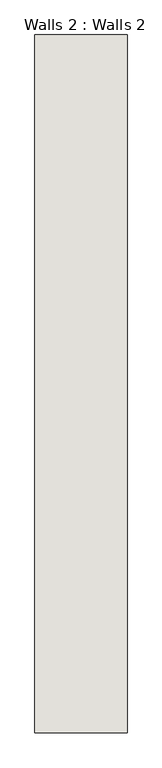
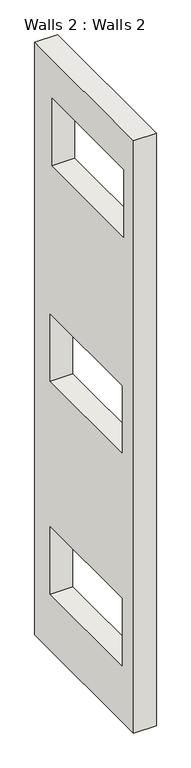
"""IFC4 building model written with IfcOpenShell, lengths in millimetres: wall geometry, Walls 2 : Walls 2."""

from ifc_helpers import new_model, si_unit, frame, origin, place, context, project, spatial, polyline, outline, extrude, source, transform, mapped, element, save


def walls_2_walls_2_0b909519(model_context):
    return source(origin(), model_context, "Body", "SweptSolid", [
        extrude(outline(polyline([(5315.00098, 12117.1681998), (5315.00098, 1394.6065085), (2379.7619319, 1394.6065085), (2379.7619319, 12117.1681998), (5315.00098, 12117.1681998)]), holes=[polyline([(4807.00098, 11414.8102851), (2673.40098, 11414.8102851), (2673.40098, 10195.6102851), (4807.00098, 10195.6102851), (4807.00098, 11414.8102851)]), polyline([(4857.80098, 7475.8655485), (2724.20098, 7475.8655485), (2724.20098, 6256.6655485), (4857.80098, 6256.6655485), (4857.80098, 7475.8655485)]), polyline([(4857.80098, 3624.7438024), (2724.20098, 3624.7438024), (2724.20098, 2405.5438024), (4857.80098, 2405.5438024), (4857.80098, 3624.7438024)])]), frame((-360.5821198, 0.0, 0.0), z_axis=(1.0, 0.0, 0.0), x_axis=(0.0, 1.0, 0.0)), (0.0, 0.0, 1.0), 387.7850165),
    ])


if __name__ == "__main__":
    model = new_model("IFC4")
    model_context = context("Model", 3, world=origin())
    ifc_project = project(units=[si_unit("LENGTHUNIT", "METRE", prefix="MILLI")], contexts=[model_context])
    site = spatial("IfcSite", under=ifc_project)
    building = spatial("IfcBuilding", under=site)
    placement = place(None, origin())
    walls_2_walls_2_shape = walls_2_walls_2_0b909519(model_context)
    element("IfcWall", 1, ObjectType="Walls 2 : Walls 2", at=placement, inside=building, context=model_context, shape_type="MappedRepresentation", body=[
        mapped(walls_2_walls_2_shape, transform((0.0, 0.0, 0.0), x_axis=(1.0, 0.0, 0.0), y_axis=(0.0, 1.0, 0.0), z_axis=(0.0, 0.0, 1.0))),
    ])
    save(model, "model.ifc")

# Revit data of these elements
# Element 1 (IfcWall, "Walls 2 : Walls 2")
#   Materials on its faces: "Default Wall"
# Materials
#   "Default Wall": colour RGB 128 128 128, transparency 0
